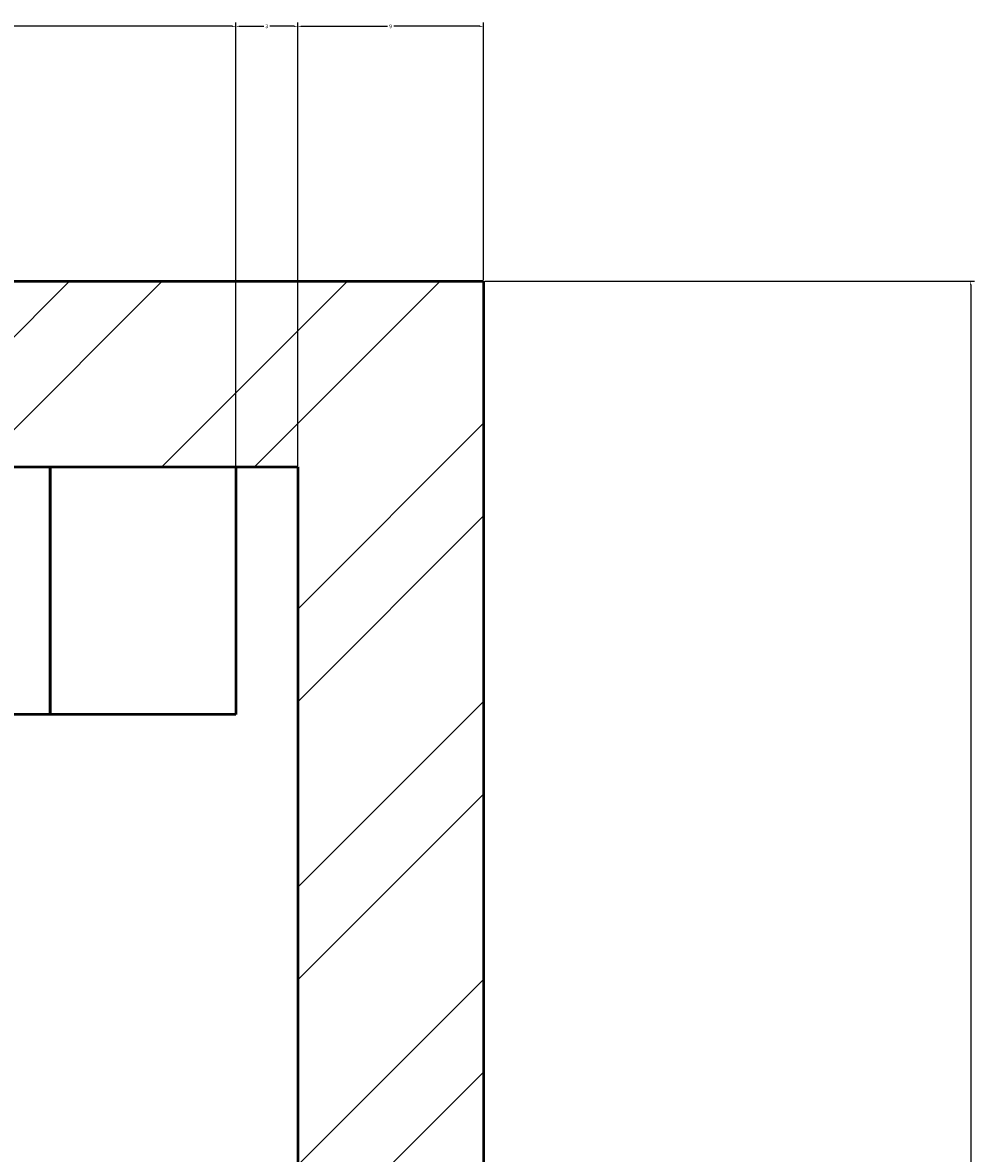
# Model space of a CAD drawing. Units: inches. Extents: x 2812 to 3051, y 1398 to 1659.
# Tile 65 of 65: x 3005 to 3051, y 1605 to 1659. Entities that reach past the tile are written whole.
import ezdxf

# ---------------------------------------------------------------- set-up
doc = ezdxf.new("R2010")
doc.units = ezdxf.units.IN
for name, color, linetype, lineweight in [('A-ANNO-DIMS', 2, 'Continuous', 18), ('S-CONC', 7, 'Continuous', 50), ('S-CONC-PATT', 8, 'Continuous', 18)]:
    doc.layers.add(name, color=color, linetype=linetype, lineweight=lineweight)
doc.styles.get("Standard").update_dxf_attribs({"font": 'arial.ttf'})
doc.dimstyles.get("Standard").update_dxf_attribs({"dimtxt": 0.18, "dimasz": 0.18, "dimexe": 0.18, "dimexo": 0.0625, "dimgap": 0.09, "dimtad": 0, "dimtih": 1, "dimtoh": 1, "dimdec": 4, "dimzin": 0, "dimdsep": 46, "dimtxsty": 'Standard', "dimcen": 0.09, "dimadec": 0, "dimazin": 0, "dimtfac": 1, "dimtdec": 4, "dimtofl": 0, "dimtmove": 0, "dimatfit": 3, "dimfxl": 1, "dimtolj": 1, "dimtzin": 0, "dimarcsym": 0})

# ---------------------------------------------------------------- blocks, each defined once
blk = doc.blocks.new('*D24')
at = {"layer": 'A-ANNO-DIMS', "color": 0, "lineweight": -2, "transparency": 16777216}
for p, q in [((2979.385, 1625.882), (2979.385, 1659.35)), ((2979.565, 1659.17), (2997.166, 1659.17)), ((3015.205, 1659.17), (2997.604, 1659.17)), ((3015.385, 1625.882), (3015.385, 1659.35))]:
    blk.add_line(p, q, dxfattribs=at)
at = {"layer": 'A-ANNO-DIMS', "color": 0, "transparency": 16777216}
for points in [[(2979.565, 1659.2), (2979.565, 1659.14), (2979.385, 1659.17)], [(3015.205, 1659.2), (3015.205, 1659.14), (3015.385, 1659.17)]]:
    blk.add_solid(points, dxfattribs=at)
at = {"layer": 'Defpoints', "color": 0, "transparency": 16777216}
for p in [(3015.385, 1659.17), (2979.385, 1625.82), (3015.385, 1625.82)]:
    blk.add_point(p, dxfattribs=at)
at = {"layer": 'A-ANNO-DIMS', "color": 0, "transparency": 16777216, "insert": (2997.385, 1659.17), "char_height": 0.18, "attachment_point": 5}
blk.add_mtext('\\A1;36', dxfattribs=at)
blk = doc.blocks.new('*D25')
at = {"layer": 'A-ANNO-DIMS', "color": 0, "lineweight": -2, "transparency": 16777216}
for p, q in [((3015.385, 1625.882), (3015.385, 1659.35)), ((3015.565, 1659.17), (3016.736, 1659.17)), ((3018.205, 1659.17), (3017.034, 1659.17)), ((3018.385, 1637.882), (3018.385, 1659.35))]:
    blk.add_line(p, q, dxfattribs=at)
at = {"layer": 'A-ANNO-DIMS', "color": 0, "transparency": 16777216}
for points in [[(3015.565, 1659.2), (3015.565, 1659.14), (3015.385, 1659.17)], [(3018.205, 1659.2), (3018.205, 1659.14), (3018.385, 1659.17)]]:
    blk.add_solid(points, dxfattribs=at)
at = {"layer": 'Defpoints', "color": 0, "transparency": 16777216}
for p in [(3018.385, 1659.17), (3018.385, 1637.82), (3015.385, 1625.82)]:
    blk.add_point(p, dxfattribs=at)
at = {"layer": 'A-ANNO-DIMS', "color": 0, "transparency": 16777216, "insert": (3016.885, 1659.17), "char_height": 0.18, "attachment_point": 5}
blk.add_mtext('\\A1;3', dxfattribs=at)
blk = doc.blocks.new('*D26')
at = {"layer": 'A-ANNO-DIMS', "color": 0, "lineweight": -2, "transparency": 16777216}
for p, q in [((3018.385, 1637.882), (3018.385, 1659.35)), ((3018.565, 1659.17), (3022.736, 1659.17)), ((3027.205, 1659.17), (3023.034, 1659.17)), ((3027.385, 1646.882), (3027.385, 1659.35))]:
    blk.add_line(p, q, dxfattribs=at)
at = {"layer": 'A-ANNO-DIMS', "color": 0, "transparency": 16777216}
for points in [[(3018.565, 1659.2), (3018.565, 1659.14), (3018.385, 1659.17)], [(3027.205, 1659.2), (3027.205, 1659.14), (3027.385, 1659.17)]]:
    blk.add_solid(points, dxfattribs=at)
at = {"layer": 'Defpoints', "color": 0, "transparency": 16777216}
for p in [(3027.385, 1659.17), (3027.385, 1646.82), (3018.385, 1637.82)]:
    blk.add_point(p, dxfattribs=at)
at = {"layer": 'A-ANNO-DIMS', "color": 0, "transparency": 16777216, "insert": (3022.885, 1659.17), "char_height": 0.18, "attachment_point": 5}
blk.add_mtext('\\A1;9', dxfattribs=at)
blk = doc.blocks.new('*D35')
at = {"layer": 'A-ANNO-DIMS', "color": 0, "lineweight": -2, "transparency": 16777216}
for p, q in [((3027.447, 1646.82), (3051.178, 1646.82)), ((3050.998, 1646.64), (3050.998, 1599.002)), ((3050.998, 1551), (3050.998, 1598.638)), ((3027.447, 1550.82), (3051.178, 1550.82))]:
    blk.add_line(p, q, dxfattribs=at)
at = {"layer": 'A-ANNO-DIMS', "color": 0, "transparency": 16777216}
for points in [[(3050.968, 1646.64), (3051.028, 1646.64), (3050.998, 1646.82)], [(3050.968, 1551), (3051.028, 1551), (3050.998, 1550.82)]]:
    blk.add_solid(points, dxfattribs=at)
at = {"layer": 'Defpoints', "color": 0, "transparency": 16777216}
for p in [(3027.385, 1646.82), (3050.998, 1646.82), (3027.385, 1550.82)]:
    blk.add_point(p, dxfattribs=at)
at = {"layer": 'A-ANNO-DIMS', "color": 0, "transparency": 16777216, "insert": (3050.998, 1598.82), "char_height": 0.18, "attachment_point": 5}
blk.add_mtext('\\A1;96', dxfattribs=at)

msp = doc.modelspace()

# ---------------------------------------------------------------- hatches: boundary and pattern name
at = {"layer": 'S-CONC-PATT'}
h = msp.add_hatch(dxfattribs=at)
h.set_pattern_fill('ANSI32', color=256)
h.paths.add_polyline_path([(3027.3849, 1646.82), (2835.3849, 1646.82), (2835.3849, 1603.2296), (2844.3849, 1603.2296), (2844.3849, 1637.82), (3018.3849, 1637.82), (3018.3849, 1602.5441), (3027.3849, 1602.5441)])
h.paths.add_polyline_path([(2844.3849, 1594.2296), (2835.3849, 1594.2296), (2835.3849, 1550.82), (3027.3849, 1550.82), (3027.3849, 1593.5441), (3018.3849, 1593.5441), (3018.3849, 1559.82), (2844.3849, 1559.82)])
h.paths.add_polyline_path([(2844.3849, 1482.0354), (2835.3849, 1482.0354), (2835.3849, 1463.4959), (2844.3849, 1463.4959)])
h.paths.add_polyline_path([(2844.3849, 1461.4959), (2835.3849, 1461.4959), (2835.3849, 1416.0354), (2844.3849, 1416.0354)])
h.paths.add_polyline_path([(3027.3849, 1482.0354), (3018.3849, 1482.0354), (3018.3849, 1463.2854), (3027.3849, 1463.2854)])
h.paths.add_polyline_path([(3027.3849, 1461.2854), (3018.3849, 1461.2854), (3018.3849, 1416.0354), (3027.3849, 1416.0354)])
h.paths.add_polyline_path([(2961.3849, 1448.4738), (2952.3849, 1448.4738), (2952.3849, 1416.0354), (2961.3849, 1416.0354)])
h.paths.add_polyline_path([(2961.3849, 1462.3026), (2952.3849, 1462.3026), (2952.3849, 1450.4738), (2961.3849, 1450.4738)])
h.paths.add_polyline_path([(2961.3849, 1472.0354), (2952.3849, 1472.0354), (2952.3849, 1462.3026), (2961.3849, 1462.3026)])

# ---------------------------------------------------------------- linework, layer by layer
at = {"layer": 'S-CONC'}
for p, q in [((2835.3849, 1646.82), (3027.3849, 1646.82)), ((3027.3849, 1646.82), (3027.3849, 1550.82)), ((2844.3849, 1637.82), (3018.3849, 1637.82)), ((2997.3849, 1637.82), (3006.3849, 1637.82)), ((3006.3849, 1637.82), (3006.3849, 1625.82)), ((3006.3849, 1625.82), (3006.3849, 1637.82)), ((3006.3849, 1637.82), (3015.3849, 1637.82)), ((3015.3849, 1637.82), (3015.3849, 1625.82)), ((3018.3849, 1637.82), (3018.3849, 1559.82)), ((3015.3849, 1625.82), (2997.3849, 1625.82))]:
    msp.add_line(p, q, dxfattribs=at)

# ---------------------------------------------------------------- dimensions: what is measured, and where the dimension line sits
at = {"layer": 'A-ANNO-DIMS'}
for base, p1, p2, picture, middle in [((3015.3849, 1659.17), (2979.3849, 1625.82), (3015.3849, 1625.82), '*D24', (2997.3849, 1659.17)), ((3018.3849, 1659.17), (3015.3849, 1625.82), (3018.3849, 1637.82), '*D25', (3016.8849, 1659.17)), ((3027.3849, 1659.17), (3018.3849, 1637.82), (3027.3849, 1646.82), '*D26', (3022.8849, 1659.17))]:
    dim = msp.add_linear_dim(base=base, p1=p1, p2=p2, dimstyle='Standard', override={"dimdec": 0, "dimlfac": 1, "dimrnd": 0, "dimzin": 0, "dimdsep": 46, "dimlunit": 2}, dxfattribs=at)
    dim.commit()
    dim.dimension.update_dxf_attribs({"geometry": picture, "text_midpoint": middle})
dim = msp.add_linear_dim(base=(3050.998, 1646.82), p1=(3027.3849, 1550.82), p2=(3027.3849, 1646.82), angle=90, dimstyle='Standard', override={"dimdec": 0, "dimlfac": 1, "dimrnd": 0, "dimzin": 0, "dimdsep": 46, "dimlunit": 2}, dxfattribs=at)
dim.commit()
dim.dimension.update_dxf_attribs({"geometry": '*D35', "text_midpoint": (3050.998, 1598.82)})

doc.saveas('drawing.dxf')
